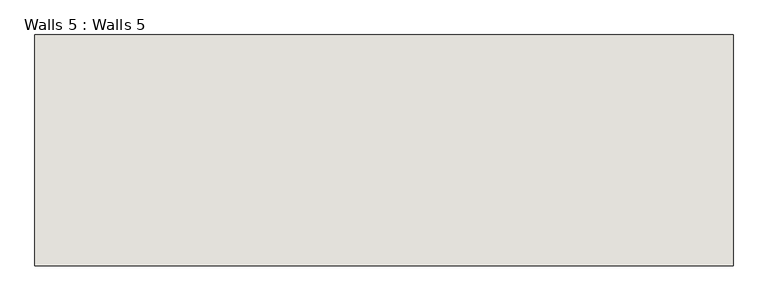
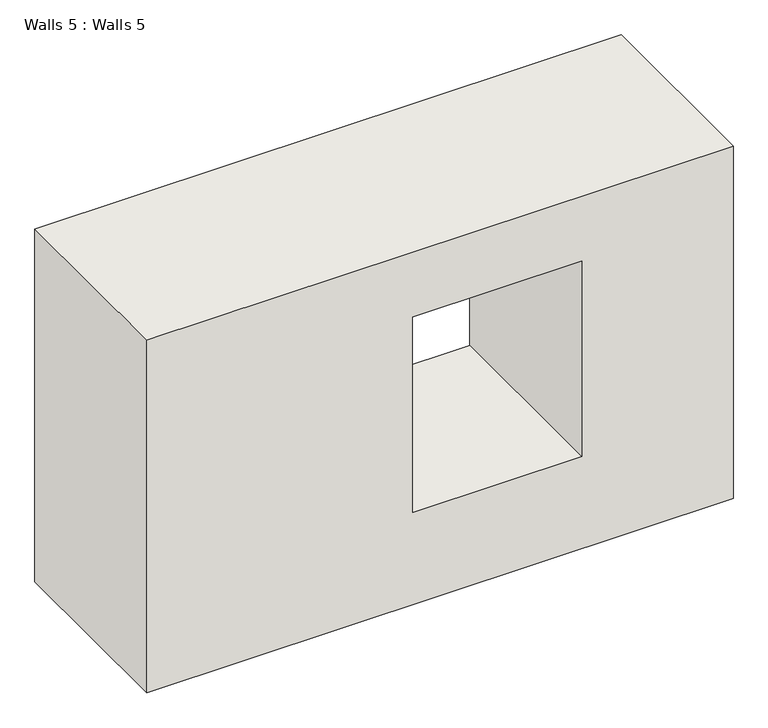
"""IFC4 building model written with IfcOpenShell, lengths in millimetres: wall geometry, Walls 5 : Walls 5."""

from ifc_helpers import new_model, si_unit, frame, origin, place, context, project, spatial, polyline, outline, extrude, source, transform, mapped, element, save


def walls_5_walls_5_db9c16c0(model_context):
    return source(origin(), model_context, "Body", "SweptSolid", [
        extrude(outline(polyline([(2327.8881187, -4840.8019361), (2327.8881187, -8498.4019361), (0.0, -8498.4019361), (0.0, -4840.8019361), (2327.8881187, -4840.8019361)]), holes=[polyline([(1898.65, -5785.3519361), (609.6, -5785.3519361), (609.6, -6839.4519361), (1898.65, -6839.4519361), (1898.65, -5785.3519361)])]), frame((0.0, -499.050374, 0.0), z_axis=(0.0, 1.0, 0.0), x_axis=(0.0, 0.0, 1.0)), (0.0, 0.0, 1.0), 1208.3940827),
    ])


if __name__ == "__main__":
    model = new_model("IFC4")
    model_context = context("Model", 3, world=origin())
    ifc_project = project(units=[si_unit("LENGTHUNIT", "METRE", prefix="MILLI")], contexts=[model_context])
    site = spatial("IfcSite", under=ifc_project)
    building = spatial("IfcBuilding", under=site)
    placement = place(None, origin())
    walls_5_walls_5_shape = walls_5_walls_5_db9c16c0(model_context)
    element("IfcWall", 1, ObjectType="Walls 5 : Walls 5", at=placement, inside=building, context=model_context, shape_type="MappedRepresentation", body=[
        mapped(walls_5_walls_5_shape, transform((0.0, 0.0, 0.0), x_axis=(1.0, 0.0, 0.0), y_axis=(0.0, 1.0, 0.0), z_axis=(0.0, 0.0, 1.0))),
    ])
    save(model, "model.ifc")

# Revit data of these elements
# Element 1 (IfcWall, "Walls 5 : Walls 5")
#   Materials on its faces: "Default Wall"
# Materials
#   "Default Wall": colour RGB 80 80 80, transparency 0
